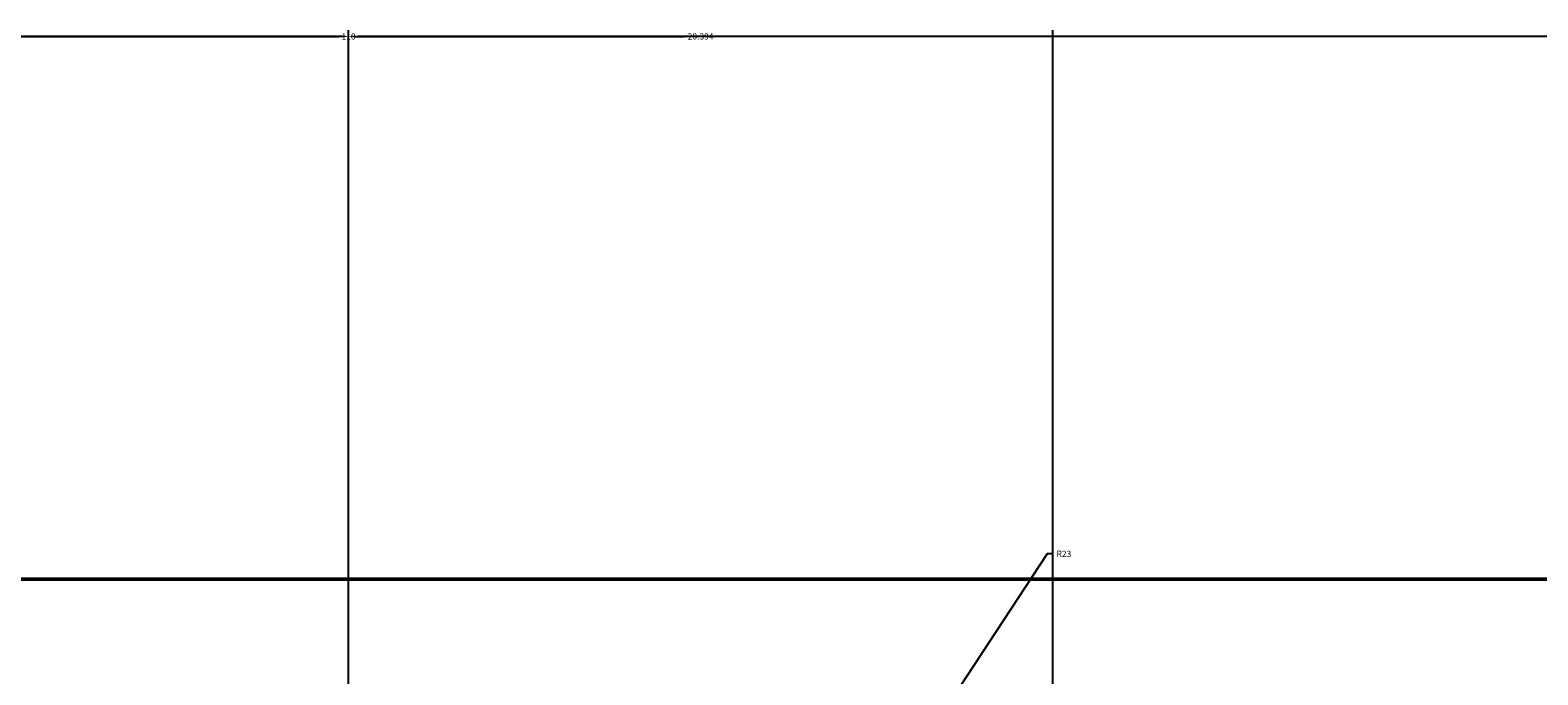
# Model space of a CAD drawing. Units: inches. Extents: x -14 to 108, y -9 to 83.
# Tile 12 of 13: x 38 to 82, y 64 to 83. Entities that reach past the tile are written whole.
import ezdxf

# ---------------------------------------------------------------- set-up
doc = ezdxf.new("R2010")
doc.units = ezdxf.units.IN
doc.header["$MEASUREMENT"] = 0
doc.layers.add('M-DIMS', color=2, linetype='Continuous', lineweight=18)
doc.layers.add('M-OUTL', color=7, linetype='Continuous', lineweight=50)
doc.styles.get("Standard").update_dxf_attribs({"font": 'arial.ttf'})
doc.dimstyles.get("Standard").update_dxf_attribs({"dimtxt": 0.18, "dimasz": 0.18, "dimexe": 0.18, "dimexo": 0.0625, "dimgap": 0.09, "dimtad": 0, "dimtih": 1, "dimtoh": 1, "dimzin": 0, "dimdsep": 46, "dimtxsty": 'Standard', "dimcen": 0.09, "dimadec": 0, "dimazin": 0, "dimtfac": 1, "dimtofl": 0, "dimtmove": 0, "dimatfit": 3, "dimfxl": 1, "dimtolj": 1, "dimtzin": 0, "dimarcsym": 0})

# ---------------------------------------------------------------- blocks, each defined once
blk = doc.blocks.new('*D4')
at = {"layer": 'Defpoints', "color": 0, "transparency": 16777216}
for p in [(102.098, 82.834), (-7.902, 67.119), (102.098, 67.119)]:
    blk.add_point(p, dxfattribs=at)
at = {"layer": 'M-DIMS', "color": 0, "lineweight": -2, "transparency": 16777216}
for p, q in [((-7.902, 67.182), (-7.902, 83.014)), ((102.098, 67.182), (102.098, 83.014)), ((-7.722, 82.834), (46.818, 82.834)), ((101.918, 82.834), (47.378, 82.834))]:
    blk.add_line(p, q, dxfattribs=at)
at = {"layer": 'M-DIMS', "color": 0, "transparency": 16777216}
for points in [[(-7.722, 82.864), (-7.722, 82.804), (-7.902, 82.834)], [(101.918, 82.864), (101.918, 82.804), (102.098, 82.834)]]:
    blk.add_solid(points, dxfattribs=at)
at = {"layer": 'M-DIMS', "color": 0, "transparency": 16777216, "insert": (47.098, 82.834), "char_height": 0.18, "attachment_point": 5}
blk.add_mtext('\\A1;110', dxfattribs=at)
blk = doc.blocks.new('*D15')
at = {"layer": 'Defpoints', "color": 0, "transparency": 16777216}
for p in [(47.098, 82.834), (47.098, 60.119), (26.462, 55.756)]:
    blk.add_point(p, dxfattribs=at)
at = {"layer": 'M-DIMS', "color": 0, "lineweight": -2, "transparency": 16777216}
for p, q in [((26.462, 55.818), (26.462, 83.014)), ((47.098, 60.182), (47.098, 83.014)), ((26.642, 82.834), (36.315, 82.834)), ((46.918, 82.834), (37.245, 82.834))]:
    blk.add_line(p, q, dxfattribs=at)
at = {"layer": 'M-DIMS', "color": 0, "transparency": 16777216}
for points in [[(26.642, 82.864), (26.642, 82.804), (26.462, 82.834)], [(46.918, 82.864), (46.918, 82.804), (47.098, 82.834)]]:
    blk.add_solid(points, dxfattribs=at)
at = {"layer": 'M-DIMS', "color": 0, "transparency": 16777216, "insert": (36.78, 82.834), "char_height": 0.18, "attachment_point": 5}
blk.add_mtext('\\A1;20.636', dxfattribs=at)
blk = doc.blocks.new('*D22')
at = {"layer": 'Defpoints', "color": 0, "transparency": 16777216}
for p in [(67.492, 82.834), (47.098, 60.119), (67.492, 47.754)]:
    blk.add_point(p, dxfattribs=at)
at = {"layer": 'M-DIMS', "color": 0, "lineweight": -2, "transparency": 16777216}
for p, q in [((47.098, 60.182), (47.098, 83.014)), ((67.492, 47.817), (67.492, 83.014)), ((47.278, 82.834), (56.83, 82.834)), ((67.312, 82.834), (57.76, 82.834))]:
    blk.add_line(p, q, dxfattribs=at)
at = {"layer": 'M-DIMS', "color": 0, "transparency": 16777216}
for points in [[(47.278, 82.864), (47.278, 82.804), (47.098, 82.834)], [(67.312, 82.864), (67.312, 82.804), (67.492, 82.834)]]:
    blk.add_solid(points, dxfattribs=at)
at = {"layer": 'M-DIMS', "color": 0, "transparency": 16777216, "insert": (57.295, 82.834), "char_height": 0.18, "attachment_point": 5}
blk.add_mtext('\\A1;20.394', dxfattribs=at)
blk = doc.blocks.new('*D30')
at = {"layer": 'Defpoints', "color": 0, "transparency": 16777216}
for p in [(59.745, 56.33), (47.098, 37.119)]:
    blk.add_point(p, dxfattribs=at)
at = {"layer": 'M-DIMS', "color": 0, "lineweight": -2, "transparency": 16777216}
for p, q in [((67.333, 67.856), (59.844, 56.48)), ((67.513, 67.856), (67.333, 67.856)), ((47.008, 37.119), (47.188, 37.119)), ((47.098, 37.029), (47.098, 37.209))]:
    blk.add_line(p, q, dxfattribs=at)
at = {"layer": 'M-DIMS', "color": 0, "transparency": 16777216}
blk.add_solid([(59.819, 56.497), (59.869, 56.464), (59.745, 56.33)], dxfattribs=at)
at = {"layer": 'M-DIMS', "color": 0, "transparency": 16777216, "insert": (67.818, 67.856), "char_height": 0.18, "attachment_point": 5}
blk.add_mtext('\\A1;R23', dxfattribs=at)

msp = doc.modelspace()

# ---------------------------------------------------------------- linework, layer by layer
at = {"layer": 'M-OUTL'}
msp.add_lwpolyline([(82.0979, 67.1193), (12.0979, 67.1193)], dxfattribs=at)

# ---------------------------------------------------------------- dimensions: what is measured, and where the dimension line sits
at = {"layer": 'M-DIMS'}
for base, p1, p2, override, picture, middle in [((102.0979, 82.8343), (-7.9021, 67.1193), (102.0979, 67.1193), {"dimdec": 0, "dimlfac": 1, "dimrnd": 0, "dimzin": 0, "dimdsep": 46, "dimlunit": 2}, '*D4', (47.0979, 82.8343)), ((47.0979, 82.8343), (26.4616, 55.7556), (47.0979, 60.1193), {"dimdec": 3, "dimlfac": 1, "dimrnd": 0, "dimzin": 0, "dimdsep": 46, "dimlunit": 2}, '*D15', (36.7798, 82.8343)), ((67.4915, 82.8343), (47.0979, 60.1193), (67.4915, 47.7542), {"dimdec": 3, "dimlfac": 1, "dimrnd": 0, "dimzin": 0, "dimdsep": 46, "dimlunit": 2}, '*D22', (57.2947, 82.8343))]:
    dim = msp.add_linear_dim(base=base, p1=p1, p2=p2, dimstyle='Standard', override=override, dxfattribs=at)
    dim.commit()
    dim.dimension.update_dxf_attribs({"geometry": picture, "text_midpoint": middle})
dim = msp.add_radius_dim(center=(47.0979, 37.1193), mpoint=(59.745, 56.33), dimstyle='Standard', override={"dimdec": 0, "dimlfac": 1, "dimrnd": 0, "dimzin": 0, "dimdsep": 46, "dimlunit": 2}, dxfattribs=at)
dim.commit()
dim.dimension.update_dxf_attribs({"geometry": '*D30', "text_midpoint": (67.8183, 67.8564), "dimtype": 164})

doc.saveas('drawing.dxf')
